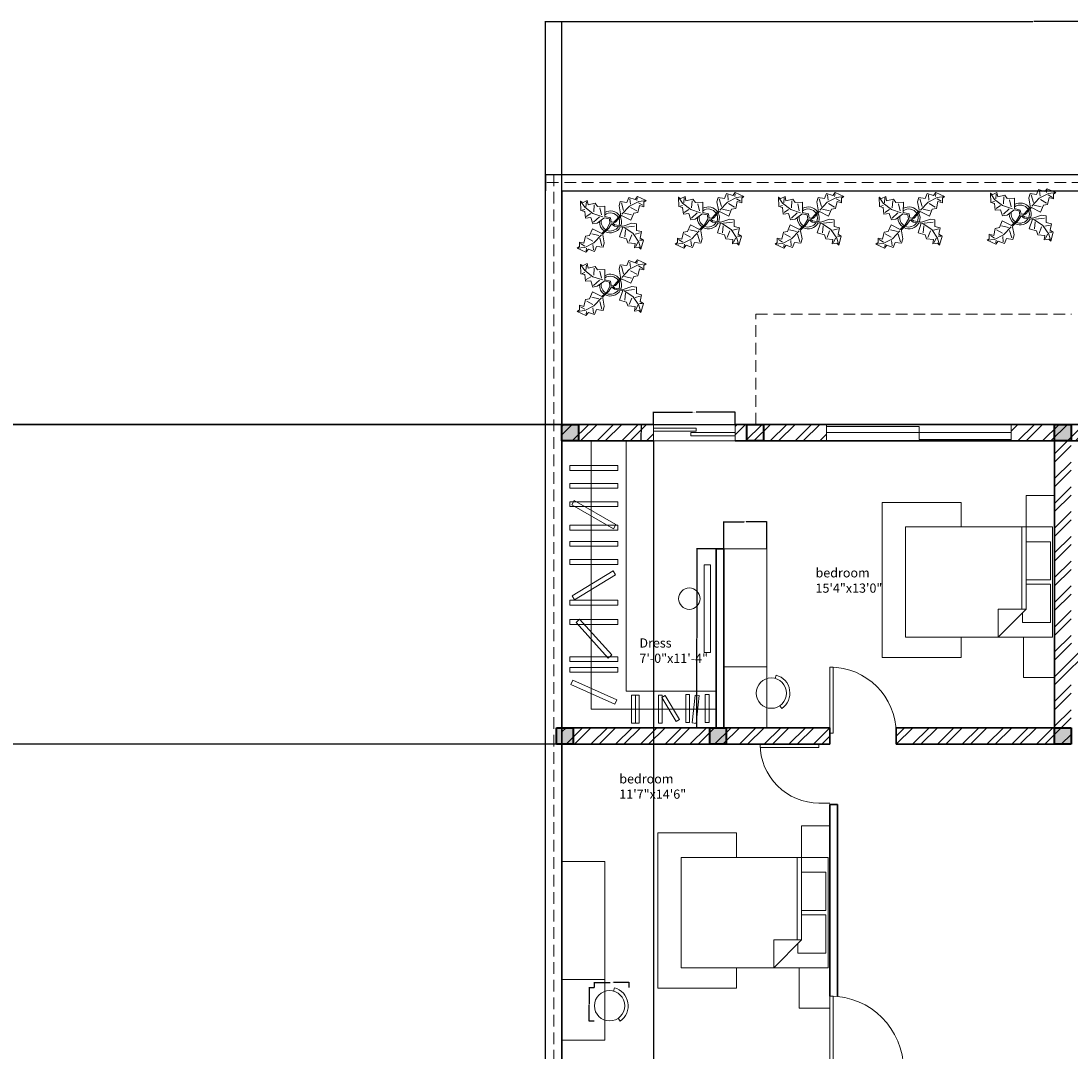
# Model space of a CAD drawing. Units: inches. Extents: x 19613 to 21413, y 12082 to 13202.
# Tile 8 of 9: x 20513 to 21084, y 12641 to 13202. Entities that reach past the tile are written whole.
import ezdxf

# ---------------------------------------------------------------- set-up
doc = ezdxf.new("R2010")
doc.units = ezdxf.units.IN
doc.linetypes.add('HIDDEN', pattern=[9.525, 6.35, -3.175])
for name, color, linetype, lineweight in [('A-ANNO-DIMS', 2, 'Continuous', 18), ('A-AREA-IDEN', 7, 'Continuous', 18), ('A-COLS', 7, 'Continuous', 40), ('A-COLS-PATT', 6, 'Continuous', 13), ('A-DOOR', 3, 'Continuous', 18), ('A-FLOR-CASE', 9, 'Continuous', 18), ('A-FLOR-HIDN', 8, 'HIDDEN', 13), ('A-FURN', 8, 'Continuous', 18), ('A-GLAZ', 4, 'Continuous', 18), ('A-WALL', 7, 'Continuous', 35), ('A-WALL-PATT', 252, 'Continuous', 13), ('C-PROP', 7, 'Continuous', 25), ('C-PROP-HIDN', 8, 'HIDDEN', 13), ('L-PLNT', 116, 'Continuous', 18)]:
    doc.layers.add(name, color=color, linetype=linetype, lineweight=lineweight)
doc.styles.get("Standard").update_dxf_attribs({"font": 'arial.ttf'})
doc.dimstyles.get("Standard").update_dxf_attribs({"dimtxt": 0.18, "dimasz": 0.18, "dimexe": 0.18, "dimexo": 0.0625, "dimgap": 0.09, "dimtad": 0, "dimtih": 1, "dimtoh": 1, "dimdec": 4, "dimzin": 0, "dimdsep": 46, "dimtxsty": 'Standard', "dimcen": 0.09, "dimadec": 0, "dimazin": 0, "dimtfac": 1, "dimtdec": 4, "dimtofl": 0, "dimtmove": 0, "dimatfit": 3, "dimfxl": 1, "dimtolj": 1, "dimtzin": 0, "dimarcsym": 0})

# ---------------------------------------------------------------- blocks, each defined once
blk = doc.blocks.new('*U4')
for p, q in [((0, 0), (0, -6)), ((36, 0), (36, -6))]:
    blk.add_line(p, q)
blk.add_lwpolyline([(0, 0), (0, 36), (1.75, 36), (1.75, 0)], close=True)
blk.add_arc((0, 0), 36, 0, 90)
blk = doc.blocks.new('Bed - Queen')
for p, q in [((0, -80.00003), (0, 0)), ((0, 0), (59.99999, 0)), ((59.99999, 0), (59.99999, -80.00003)), ((7.99999, -1.2), (28.79998, -1.2)), ((7.99999, -14.4), (7.99999, -1.2)), ((28.79998, -1.2), (28.79998, -14.4)), ((31.19999, -1.2), (51.99999, -1.2)), ((31.19999, -14.4), (31.19999, -1.2)), ((51.99999, -1.2), (51.99999, -16.4)), ((0, -14.4), (44.8, -14.4)), ((44.8, -16.8), (0, -16.8)), ((59.99999, -29.6), (44.8, -14.4)), ((44.8, -14.4), (44.8, -29.6)), ((51.99999, -16.4), (46.79936, -16.4)), ((44.8, -29.6), (59.99999, -29.6)), ((59.99999, -80.00003), (0, -80.00003))]:
    blk.add_line(p, q)
blk = doc.blocks.new('*U6')
for p, q in [((0, 0), (0, -6)), ((40, 0), (40, -6))]:
    blk.add_line(p, q)
blk.add_lwpolyline([(0, 0), (0, 40), (1.75, 40), (1.75, 0)], close=True)
blk.add_arc((0, 0), 40, 0, 90)
blk = doc.blocks.new('Plant - Rubber or Philodendron')
for p, q in [((-16.2005, 11.4774), (-13.9899, 8.1064)), ((-16.2005, 11.4774), (-14.8639, 10.7964)), ((-16.0159, 6.3329), (-16.2005, 11.4774)), ((-14.8639, 10.7964), (-12.6195, 11.8975)), ((-12.6195, 11.8975), (-12.1909, 9.4345)), ((8.8871, 10.7908), (9.9809, 13.4933)), ((9.9809, 13.4933), (13.3837, 12.301)), ((10.5828, 12.6946), (10.8893, 9.7953)), ((13.3837, 12.301), (14.68, 13.9039)), ((14.5816, 13.2037), (14.3848, 11.8033)), ((14.68, 13.9039), (19.3848, 11.8146)), ((19.3848, 11.8146), (15.3859, 11.3055)), ((19.3848, 11.8146), (18.1868, 10.9119)), ((-14.0069, 5.8704), (-16.0159, 6.3329)), ((-15.3434, 6.5514), (-13.9984, 6.9884)), ((-13.5868, 2.2894), (-14.0069, 5.8704)), ((-13.9899, 8.1064), (-9.5434, 4.7185)), ((-13.3174, 8.325), (-13.0735, 11.0065)), ((-12.1909, 9.4345), (-8.3829, 10.3)), ((-8.8369, 9.409), (-9.0894, 5.6095)), ((-8.3829, 10.3), (-7.0549, 8.501)), ((-7.0549, 8.501), (-3.0284, 8.6941)), ((-4.8529, 4.012), (-5.7184, 7.82)), ((-3.0284, 8.6941), (-3.0709, 3.1041)), ((4.6914, 8.8812), (5.3859, 11.2828)), ((4.6914, 8.8812), (5.5014, 4.4831)), ((5.3859, 11.2828), (8.8871, 10.7908)), ((5.9878, 10.4842), (7.1971, 6.3869)), ((10.3916, 8.7942), (6.2847, 4.4028)), ((15.3859, 11.3055), (10.3916, 8.7942)), ((14.2977, 6.1031), (10.9934, 7.9956)), ((15.7909, 9.1065), (14.8995, 5.3044)), ((15.2875, 10.6053), (17.5907, 9.2105)), ((18.1925, 8.4119), (15.7909, 9.1065)), ((18.1868, 10.9119), (18.1925, 8.4119)), ((-10.6784, 2.491), (-13.5868, 2.2894)), ((-13.1329, 3.1804), (-10.6614, 4.727)), ((-9.5858, -0.8715), (-10.6784, 2.491)), ((-9.5434, 4.7185), (-4.1917, 2.9888)), ((-9.1318, 0.0195), (-5.9793, 2.9025)), ((-7.1228, -0.443), (-3.5248, 2.2131)), ((-3.5248, 2.2131), (-3.3011, 2.4355)), ((-3.3011, 2.4355), (-0.5306, 1.7947)), ((-3.0709, 3.1041), (0.0797, 2.3163)), ((-0.5306, 1.7947), (-0.2255, -0.5527)), ((-0.5306, 1.7947), (-0.5306, 1.7947)), ((0.0797, 2.3163), (0.4866, -0.031)), ((0.4866, -0.031), (2.1141, 0.2298)), ((2.1141, 0.2298), (5.4346, 3.9146)), ((6.1032, 3.6844), (2.8262, -0.031)), ((5.4346, 3.9146), (5.5014, 4.4831)), ((11.1089, 1.1958), (6.1032, 3.6844)), ((7.7005, 4.8881), (11.5025, 3.9967)), ((12.7005, 4.8994), (11.1089, 1.1958)), ((14.8995, 5.3044), (12.7005, 4.8994)), ((-11.3237, -7.2629), (-9.7321, -3.5593)), ((-9.7321, -3.5593), (-4.7264, -6.0479)), ((-7.1228, -0.443), (-9.5858, -0.8715)), ((-2.019, -3.6148), (-4.7264, -6.0479)), ((-4.0579, -6.2781), (-0.9375, -3.1608)), ((-2.019, -3.6148), (-0.2255, -0.5527)), ((-0.9375, -3.1608), (0.5883, -0.8135)), ((0.5883, -0.8135), (2.2447, -2.0916)), ((2.8262, -0.031), (1.3003, -0.5527)), ((1.3003, -0.5527), (2.4193, -1.4655)), ((2.2447, -2.0916), (6.7108, -2.6626)), ((2.4193, -1.4655), (6.895, -2.1175)), ((4.943, -7.9659), (6.7108, -2.6626)), ((11.6605, -0.5413), (6.895, -2.1175)), ((12.3677, -6.1981), (7.219, -2.6772)), ((8.125, -4.0768), (7.7715, -7.9659)), ((8.3544, -2.7453), (13.1973, -2.1704)), ((11.6605, -0.5413), (14.1354, -0.8948)), ((14.1354, -0.8948), (14.1354, -4.4304)), ((14.1354, -4.4304), (16.9638, -5.1375)), ((16.9638, -5.1375), (16.2567, -8.673)), ((-16.8157, -10.7754), (-14.4141, -11.4699)), ((-16.8101, -13.2754), (-16.8157, -10.7754)), ((-14.4141, -11.4699), (-13.5228, -7.6679)), ((-14.0091, -13.669), (-9.0148, -11.1577)), ((-13.5228, -7.6679), (-11.3237, -7.2629)), ((-12.921, -8.4665), (-9.6166, -10.359)), ((-6.3237, -7.2516), (-10.1257, -6.3602)), ((-9.0148, -11.1577), (-4.9047, -6.8122)), ((-4.611, -12.8477), (-5.8203, -8.7504)), ((-4.1246, -6.8466), (-4.0579, -6.2781)), ((-3.3146, -11.2447), (-4.1246, -6.8466)), ((-3.3146, -11.2447), (-4.0092, -13.6463)), ((8.8321, -9.0266), (4.943, -7.9659)), ((9.5392, -11.1479), (8.8321, -9.0266)), ((13.4283, -11.5015), (9.5392, -11.1479)), ((10.2463, -10.4408), (11.6605, -6.9053)), ((15.5496, -10.7943), (12.3677, -6.1981)), ((16.2567, -5.8446), (13.4283, -6.5517)), ((14.8425, -10.7943), (13.7819, -13.2692)), ((16.6103, -14.6834), (15.5496, -10.7943)), ((17.3174, -9.7337), (15.9032, -9.7337)), ((16.2567, -8.673), (18.0245, -9.7337)), ((18.0245, -9.7337), (16.6103, -14.6834)), ((-18.008, -14.1781), (-16.8101, -13.2754)), ((-18.008, -14.1781), (-14.0091, -13.669)), ((-13.3032, -16.2674), (-18.008, -14.1781)), ((-13.9107, -12.9688), (-16.2139, -11.574)), ((-12.0069, -14.6645), (-13.3032, -16.2674)), ((-13.2048, -15.5672), (-13.008, -14.1668)), ((-8.6042, -15.8568), (-12.0069, -14.6645)), ((-9.206, -15.0581), (-9.5126, -12.1588)), ((-7.5103, -13.1543), (-8.6042, -15.8568)), ((-4.0092, -13.6463), (-7.5103, -13.1543)), ((13.0748, -13.9763), (13.4283, -11.5015)), ((15.5496, -13.6228), (13.0748, -13.9763)), ((16.6103, -14.6834), (15.5496, -13.6228))]:
    blk.add_line(p, q)
for centre, radius, start, end in [((0, 0), 6.1275, 34.37569, 120.1028), ((0.0308, 0.1664), 6, 178.6147, 235.1169), ((0.0308, 0.1664), 5, 168.1647, 238.6725), ((-0.0601, -0.2075), 5.2461, 33.82192, 124.9414), ((-0.2664, 0.1682), 5.2775, 338.4094, 20.03007), ((-0.098, 0.1364), 6.1288, 341.2017, 26.09184), ((-0.0234, 0.3825), 6.1492, 242.5812, 331.2714), ((-0.1102, 0.4886), 5.2883, 247.3711, 327.472)]:
    blk.add_arc(centre, radius, start, end)
blk = doc.blocks.new('*U16')
for p, q in [((0, 0), (0, 6)), ((32, 0), (32, 6))]:
    blk.add_line(p, q)
blk.add_lwpolyline([(0, 0), (0, -32), (1.75, -32), (1.75, 0)], close=True)
blk.add_arc((0, 0), 32, 270, 0)
blk = doc.blocks.new('COL-9x9')
for p, q in [((0, 9), (9, 9)), ((0, 0), (0, 9)), ((9, 9), (9, 0)), ((9, 0), (0, 0))]:
    blk.add_line(p, q)
blk = doc.blocks.new('CLOSET-L-RAIL')
for p, q in [((11.57, 153.64), (11.57, 7.7)), ((30.65, 153.64), (30.65, 17.54)), ((30.65, 17.54), (79.7, 17.54)), ((11.57, 7.7), (79.7, 7.7))]:
    blk.add_line(p, q)
for points in [[(0, 140.24), (26.12, 140.24), (26.12, 137.64), (0, 137.64)], [(0, 130.54), (26.12, 130.54), (26.12, 127.95), (0, 127.95)], [(0, 120.52), (26.12, 120.52), (26.12, 117.92), (0, 117.92)], [(2.39, 121.15), (25.03, 108.13), (23.74, 105.88), (1.09, 118.9)], [(0, 107.73), (26.12, 107.73), (26.12, 105.13), (0, 105.13)], [(0, 98.91), (26.12, 98.91), (26.12, 96.32), (0, 96.32)], [(0, 89.07), (26.12, 89.07), (26.12, 86.48), (0, 86.48)], [(1.22, 69.39), (23.56, 82.95), (24.9, 80.73), (2.57, 67.18)], [(0, 66.96), (26.12, 66.96), (26.12, 64.37), (0, 64.37)], [(0, 56.45), (26.12, 56.45), (26.12, 53.86), (0, 53.86)], [(5.27, 56.6), (22.78, 37.21), (20.85, 35.47), (3.35, 54.86)], [(0, 36.27), (26.12, 36.27), (26.12, 33.68), (0, 33.68)], [(0, 30.47), (26.12, 30.47), (26.12, 27.88), (0, 27.88)], [(1.67, 23.53), (25.51, 12.85), (24.45, 10.49), (0.61, 21.17)], [(35.67, 0.07), (33.61, 0.07), (33.61, 15.33), (35.67, 15.33)], [(37.73, 0.07), (35.67, 0.07), (35.67, 15.33), (37.73, 15.33)], [(50.3, 0.07), (48.24, 0.07), (48.24, 15.33), (50.3, 15.33)], [(59.69, 2.02), (57.92, 0.97), (50.13, 14.1), (51.9, 15.15)], [(65.15, 0.43), (63.09, 0.43), (63.09, 15.69), (65.15, 15.69)], [(68.26, 15.4), (70.31, 15.18), (68.65, 0), (66.6, 0.22)], [(75.77, 0.43), (73.71, 0.43), (73.71, 15.69), (75.77, 15.69)]]:
    blk.add_lwpolyline(points, close=True)
blk = doc.blocks.new('WINDOW-BEDROOM-SLIDER')
for p, q in [((0, 9), (0, 0)), ((0, 9), (100.32, 9)), ((0, 0), (0, 9)), ((50.28, 7.85), (0, 7.85)), ((50.28, 4.5), (50.28, 7.85)), ((50.28, 7.85), (50.28, 4.5)), ((100.32, 9), (100.32, 0)), ((100.32, 9), (100.32, 0.84)), ((0, 4.5), (50.28, 4.5)), ((50.28, 4.5), (100.32, 4.5)), ((100.32, 4.5), (50.28, 4.5)), ((50.28, 4.5), (50.28, 0.84)), ((50.28, 0.84), (100.32, 0.84)), ((100.32, 0.84), (100.32, 0)), ((100.32, 0), (0, 0))]:
    blk.add_line(p, q)
blk = doc.blocks.new('WINDOW-DRESS-SLIDER')
for p, q in [((0, 9), (0, 0)), ((0, 9), (44.45, 9)), ((44.45, 9), (44.45, 0)), ((0, 0), (44.45, 0))]:
    blk.add_line(p, q)
for points in [[(0, 6.95), (23.27, 6.95), (23.27, 5.37), (0, 5.37)], [(44.45, 4.5), (20.22, 4.5), (20.22, 2.83), (44.45, 2.83)]]:
    blk.add_lwpolyline(points, close=True)
blk = doc.blocks.new('DESK-CHAIR-ROUND')
for p, q in [((10.85, 18.16), (10.37, 16.34)), ((13.96, 0), (12.89, 1.56))]:
    blk.add_line(p, q)
blk.add_circle((8.25, 8.37), 8.25)
blk.add_arc((8.25, 8.37), 10.13, 304.3105, 75.0908)
blk = doc.blocks.new('BEDROOM-DESK-SLIM')
for p, q in [((0, 97.32), (23.4, 97.32)), ((23.4, 97.32), (23.4, 0)), ((0, 33.03), (23.4, 33.03))]:
    blk.add_line(p, q)
blk = doc.blocks.new('BEDROOM-AREA-RUG')
for p, q in [((42.96, 84.39), (0, 84.39)), ((0, 84.39), (0, 0)), ((42.96, 71.03), (42.96, 84.39)), ((12.72, 71.03), (42.96, 71.03)), ((42.96, 0), (42.96, 11.03)), ((0, 0), (42.96, 0))]:
    blk.add_line(p, q)
blk = doc.blocks.new('*D45')
at = {"layer": 'A-ANNO-DIMS', "color": 0, "lineweight": -2, "transparency": 16777216}
for p, q in [((20825.11, 12675.88), (20825.11, 12678.83)), ((20844.01, 12675.88), (20844.01, 12678.83)), ((20825.29, 12678.65), (20833.6, 12678.65)), ((20843.83, 12678.65), (20835.51, 12678.65))]:
    blk.add_line(p, q, dxfattribs=at)
at = {"layer": 'A-ANNO-DIMS', "color": 0, "transparency": 16777216}
for points in [[(20825.29, 12678.68), (20825.29, 12678.62), (20825.11, 12678.65)], [(20843.83, 12678.68), (20843.83, 12678.62), (20844.01, 12678.65)]]:
    blk.add_solid(points, dxfattribs=at)
at = {"layer": 'Defpoints', "color": 0, "transparency": 16777216}
for p in [(20825.11, 12675.81), (20844.01, 12678.65), (20844.01, 12675.81)]:
    blk.add_point(p, dxfattribs=at)
at = {"layer": 'A-ANNO-DIMS', "color": 0, "transparency": 16777216, "insert": (20834.56, 12678.65), "char_height": 0.18, "attachment_point": 5}
blk.add_mtext('\\A1;CHAIR 19 TYP.', dxfattribs=at)
blk = doc.blocks.new('*D46')
at = {"layer": 'A-ANNO-DIMS', "color": 0, "lineweight": -2, "transparency": 16777216}
for p, q in [((20825.04, 12675.81), (20822.09, 12675.81)), ((20822.27, 12675.63), (20822.27, 12666.92)), ((20822.27, 12657.83), (20822.27, 12666.55)), ((20825.04, 12657.65), (20822.09, 12657.65))]:
    blk.add_line(p, q, dxfattribs=at)
at = {"layer": 'A-ANNO-DIMS', "color": 0, "transparency": 16777216}
for points in [[(20822.24, 12675.63), (20822.3, 12675.63), (20822.27, 12675.81)], [(20822.24, 12657.83), (20822.3, 12657.83), (20822.27, 12657.65)]]:
    blk.add_solid(points, dxfattribs=at)
at = {"layer": 'Defpoints', "color": 0, "transparency": 16777216}
for p in [(20822.27, 12675.81), (20825.11, 12675.81), (20825.11, 12657.65)]:
    blk.add_point(p, dxfattribs=at)
at = {"layer": 'A-ANNO-DIMS', "color": 0, "transparency": 16777216, "insert": (20822.27, 12666.73), "char_height": 0.18, "attachment_point": 5}
blk.add_mtext('\\A1;18 TYP.', dxfattribs=at)
blk = doc.blocks.new('*D47')
at = {"layer": 'A-ANNO-DIMS', "color": 0, "lineweight": -2, "transparency": 16777216}
for p, q in [((20895.37, 12914.6), (20880.66, 12914.6)), ((20880.84, 12914.42), (20880.84, 12866.12)), ((20880.84, 12817.46), (20880.84, 12865.75)), ((20895.37, 12817.28), (20880.66, 12817.28))]:
    blk.add_line(p, q, dxfattribs=at)
at = {"layer": 'A-ANNO-DIMS', "color": 0, "transparency": 16777216}
for points in [[(20880.81, 12914.42), (20880.87, 12914.42), (20880.84, 12914.6)], [(20880.81, 12817.46), (20880.87, 12817.46), (20880.84, 12817.28)]]:
    blk.add_solid(points, dxfattribs=at)
at = {"layer": 'Defpoints', "color": 0, "transparency": 16777216}
for p in [(20880.84, 12914.6), (20895.43, 12914.6), (20895.43, 12817.28)]:
    blk.add_point(p, dxfattribs=at)
at = {"layer": 'A-ANNO-DIMS', "color": 0, "transparency": 16777216, "insert": (20880.84, 12865.94), "char_height": 0.18, "attachment_point": 5}
blk.add_mtext('\\A1;DESK 97 TYP.', dxfattribs=at)
blk = doc.blocks.new('*D48')
at = {"layer": 'A-ANNO-DIMS', "color": 0, "lineweight": -2, "transparency": 16777216}
for p, q in [((20895.43, 12914.66), (20895.43, 12929.37)), ((20895.61, 12929.19), (20906.6, 12929.19)), ((20918.65, 12929.19), (20907.66, 12929.19)), ((20918.83, 12914.66), (20918.83, 12929.37))]:
    blk.add_line(p, q, dxfattribs=at)
at = {"layer": 'A-ANNO-DIMS', "color": 0, "transparency": 16777216}
for points in [[(20895.61, 12929.22), (20895.61, 12929.16), (20895.43, 12929.19)], [(20918.65, 12929.22), (20918.65, 12929.16), (20918.83, 12929.19)]]:
    blk.add_solid(points, dxfattribs=at)
at = {"layer": 'Defpoints', "color": 0, "transparency": 16777216}
for p in [(20918.83, 12929.19), (20895.43, 12914.6), (20918.83, 12914.6)]:
    blk.add_point(p, dxfattribs=at)
at = {"layer": 'A-ANNO-DIMS', "color": 0, "transparency": 16777216, "insert": (20907.13, 12929.19), "char_height": 0.18, "attachment_point": 5}
blk.add_mtext('\\A1;23 TYP.', dxfattribs=at)
blk = doc.blocks.new('*D63')
at = {"layer": 'A-ANNO-DIMS', "color": 0, "lineweight": -2, "transparency": 16777216}
for p, q in [((20857.28, 12982.34), (20857.28, 12989.13)), ((20857.46, 12988.95), (20878.49, 12988.95)), ((20901.55, 12988.95), (20880.52, 12988.95)), ((20901.73, 12982.34), (20901.73, 12989.13))]:
    blk.add_line(p, q, dxfattribs=at)
at = {"layer": 'A-ANNO-DIMS', "color": 0, "transparency": 16777216}
for points in [[(20857.46, 12988.98), (20857.46, 12988.92), (20857.28, 12988.95)], [(20901.55, 12988.98), (20901.55, 12988.92), (20901.73, 12988.95)]]:
    blk.add_solid(points, dxfattribs=at)
at = {"layer": 'Defpoints', "color": 0, "transparency": 16777216}
for p in [(20901.73, 12988.95), (20857.28, 12982.28), (20901.73, 12982.28)]:
    blk.add_point(p, dxfattribs=at)
at = {"layer": 'A-ANNO-DIMS', "color": 0, "transparency": 16777216, "insert": (20879.5, 12988.95), "char_height": 0.18, "attachment_point": 5}
blk.add_mtext('\\A1;SLIDER 44 TYP.', dxfattribs=at)
blk = doc.blocks.new('*D64')
at = {"layer": 'A-ANNO-DIMS', "color": 0, "lineweight": -2, "transparency": 16777216}
for p, q in [((20857.22, 12982.28), (20850.43, 12982.28)), ((20850.61, 12982.1), (20850.61, 12977.96)), ((20850.61, 12973.46), (20850.61, 12977.6)), ((20857.22, 12973.28), (20850.43, 12973.28))]:
    blk.add_line(p, q, dxfattribs=at)
at = {"layer": 'A-ANNO-DIMS', "color": 0, "transparency": 16777216}
for points in [[(20850.58, 12982.1), (20850.64, 12982.1), (20850.61, 12982.28)], [(20850.58, 12973.46), (20850.64, 12973.46), (20850.61, 12973.28)]]:
    blk.add_solid(points, dxfattribs=at)
at = {"layer": 'Defpoints', "color": 0, "transparency": 16777216}
for p in [(20850.61, 12982.28), (20857.28, 12982.28), (20857.28, 12973.28)]:
    blk.add_point(p, dxfattribs=at)
at = {"layer": 'A-ANNO-DIMS', "color": 0, "transparency": 16777216, "insert": (20850.61, 12977.78), "char_height": 0.18, "attachment_point": 5}
blk.add_mtext('\\A1;9 TYP.', dxfattribs=at)
blk = doc.blocks.new('*D85')
at = {"layer": 'A-ANNO-DIMS', "color": 0, "lineweight": -2, "transparency": 16777216}
for p, q in [((20798.43, 13118.34), (20798.43, 13201.71)), ((20798.61, 13201.53), (21063.66, 13201.53)), ((21329.25, 13201.53), (21064.21, 13201.53)), ((21329.43, 13118.34), (21329.43, 13201.71))]:
    blk.add_line(p, q, dxfattribs=at)
at = {"layer": 'A-ANNO-DIMS', "color": 0, "transparency": 16777216}
for points in [[(20798.61, 13201.56), (20798.61, 13201.5), (20798.43, 13201.53)], [(21329.25, 13201.56), (21329.25, 13201.5), (21329.43, 13201.53)]]:
    blk.add_solid(points, dxfattribs=at)
at = {"layer": 'Defpoints', "color": 0, "transparency": 16777216}
for p in [(21329.43, 13201.53), (20798.43, 13118.28), (21329.43, 13118.28)]:
    blk.add_point(p, dxfattribs=at)
at = {"layer": 'A-ANNO-DIMS', "color": 0, "transparency": 16777216, "insert": (21063.93, 13201.53), "char_height": 0.18, "attachment_point": 5}
blk.add_mtext('\\A1;531', dxfattribs=at)
blk = doc.blocks.new('*D87')
at = {"layer": 'A-ANNO-DIMS', "color": 0, "lineweight": -2, "transparency": 16777216}
for p, q in [((20218.76, 12982.28), (21412.86, 12982.28)), ((21412.68, 12982.1), (21412.68, 12697.46)), ((21412.68, 12412.46), (21412.68, 12697.1)), ((20218.76, 12412.28), (21412.86, 12412.28))]:
    blk.add_line(p, q, dxfattribs=at)
at = {"layer": 'A-ANNO-DIMS', "color": 0, "transparency": 16777216}
for points in [[(21412.65, 12982.1), (21412.71, 12982.1), (21412.68, 12982.28)], [(21412.65, 12412.46), (21412.71, 12412.46), (21412.68, 12412.28)]]:
    blk.add_solid(points, dxfattribs=at)
at = {"layer": 'Defpoints', "color": 0, "transparency": 16777216}
for p in [(20218.69, 12982.28), (21412.68, 12982.28), (20218.69, 12412.28)]:
    blk.add_point(p, dxfattribs=at)
at = {"layer": 'A-ANNO-DIMS', "color": 0, "transparency": 16777216, "insert": (21412.68, 12697.28), "char_height": 0.18, "attachment_point": 5}
blk.add_mtext('\\A1;570', dxfattribs=at)
blk = doc.blocks.new('*D89')
at = {"layer": 'A-ANNO-DIMS', "color": 0, "lineweight": -2, "transparency": 16777216}
for p, q in [((20807.37, 12808.28), (19613.26, 12808.28)), ((19613.44, 12808.1), (19613.44, 12721.46)), ((19613.44, 12634.46), (19613.44, 12721.1)), ((20807.37, 12634.28), (19613.26, 12634.28))]:
    blk.add_line(p, q, dxfattribs=at)
at = {"layer": 'A-ANNO-DIMS', "color": 0, "transparency": 16777216}
for points in [[(19613.41, 12808.1), (19613.47, 12808.1), (19613.44, 12808.28)], [(19613.41, 12634.46), (19613.47, 12634.46), (19613.44, 12634.28)]]:
    blk.add_solid(points, dxfattribs=at)
at = {"layer": 'Defpoints', "color": 0, "transparency": 16777216}
for p in [(19613.44, 12808.28), (20807.43, 12808.28), (20807.43, 12634.28)]:
    blk.add_point(p, dxfattribs=at)
at = {"layer": 'A-ANNO-DIMS', "color": 0, "transparency": 16777216, "insert": (19613.44, 12721.28), "char_height": 0.18, "attachment_point": 5}
blk.add_mtext('\\A1;174', dxfattribs=at)
blk = doc.blocks.new('*D90')
at = {"layer": 'A-ANNO-DIMS', "color": 0, "lineweight": -2, "transparency": 16777216}
for p, q in [((20807.37, 12982.28), (19613.26, 12982.28)), ((19613.44, 12982.1), (19613.44, 12895.46)), ((19613.44, 12808.46), (19613.44, 12895.1)), ((20807.37, 12808.28), (19613.26, 12808.28))]:
    blk.add_line(p, q, dxfattribs=at)
at = {"layer": 'A-ANNO-DIMS', "color": 0, "transparency": 16777216}
for points in [[(19613.41, 12982.1), (19613.47, 12982.1), (19613.44, 12982.28)], [(19613.41, 12808.46), (19613.47, 12808.46), (19613.44, 12808.28)]]:
    blk.add_solid(points, dxfattribs=at)
at = {"layer": 'Defpoints', "color": 0, "transparency": 16777216}
for p in [(19613.44, 12982.28), (20807.43, 12982.28), (20807.43, 12808.28)]:
    blk.add_point(p, dxfattribs=at)
at = {"layer": 'A-ANNO-DIMS', "color": 0, "transparency": 16777216, "insert": (19613.44, 12895.28), "char_height": 0.18, "attachment_point": 5}
blk.add_mtext('\\A1;174', dxfattribs=at)
blk = doc.blocks.new('*D98')
at = {"layer": 'A-ANNO-DIMS', "color": 0, "lineweight": -2, "transparency": 16777216}
for p, q in [((20807.43, 12982.34), (20807.43, 13201.71)), ((20807.61, 13201.53), (21063.64, 13201.53)), ((21320.25, 13201.53), (21064.22, 13201.53)), ((21320.43, 12982.34), (21320.43, 13201.71))]:
    blk.add_line(p, q, dxfattribs=at)
at = {"layer": 'A-ANNO-DIMS', "color": 0, "transparency": 16777216}
for points in [[(20807.61, 13201.56), (20807.61, 13201.5), (20807.43, 13201.53)], [(21320.25, 13201.56), (21320.25, 13201.5), (21320.43, 13201.53)]]:
    blk.add_solid(points, dxfattribs=at)
at = {"layer": 'Defpoints', "color": 0, "transparency": 16777216}
for p in [(21320.43, 13201.53), (20807.43, 12982.28), (21320.43, 12982.28)]:
    blk.add_point(p, dxfattribs=at)
at = {"layer": 'A-ANNO-DIMS', "color": 0, "transparency": 16777216, "insert": (21063.93, 13201.53), "char_height": 0.18, "attachment_point": 5}
blk.add_mtext('\\A1;513', dxfattribs=at)
blk = doc.blocks.new('*D100')
at = {"layer": 'A-ANNO-DIMS', "color": 0, "lineweight": -2, "transparency": 16777216}
for p, q in [((20807.43, 12973.22), (20807.43, 12091.85)), ((20857.28, 12973.22), (20857.28, 12091.85)), ((20807.61, 12092.03), (20831.96, 12092.03)), ((20857.1, 12092.03), (20832.75, 12092.03))]:
    blk.add_line(p, q, dxfattribs=at)
at = {"layer": 'A-ANNO-DIMS', "color": 0, "transparency": 16777216}
for points in [[(20807.61, 12092.06), (20807.61, 12092), (20807.43, 12092.03)], [(20857.1, 12092.06), (20857.1, 12092), (20857.28, 12092.03)]]:
    blk.add_solid(points, dxfattribs=at)
at = {"layer": 'Defpoints', "color": 0, "transparency": 16777216}
for p in [(20807.43, 12973.28), (20857.28, 12973.28), (20857.28, 12092.03)]:
    blk.add_point(p, dxfattribs=at)
at = {"layer": 'A-ANNO-DIMS', "color": 0, "transparency": 16777216, "insert": (20832.36, 12092.03), "char_height": 0.18, "attachment_point": 5}
blk.add_mtext('\\A1;49.85', dxfattribs=at)

msp = doc.modelspace()

# ---------------------------------------------------------------- hatches: boundary and pattern name
at = {"layer": 'A-COLS-PATT'}
h = msp.add_hatch(color=256, dxfattribs=at)
h.dxf.hatch_style = 1
h.paths.add_polyline_path([(20816.4328, 12982.279), (20807.4339, 12982.279), (20807.4339, 12973.279), (20816.4328, 12973.279)])
h.paths.add_polyline_path([(21084.4339, 12982.279), (21075.4339, 12982.279), (21075.4339, 12973.279), (21084.4339, 12973.279)])
h.paths.add_polyline_path([(21320.4339, 12982.279), (21311.4729, 12982.279), (21311.4729, 12973.279), (21320.4339, 12973.279)])
h.paths.add_polyline_path([(21320.3201, 12808.279), (21311.3201, 12808.279), (21311.3201, 12803.279), (21320.3201, 12803.279)])
h.paths.add_polyline_path([(21320.3201, 12812.279), (21311.3201, 12812.279), (21311.3201, 12808.279), (21320.3201, 12808.279)])
h.paths.add_polyline_path([(21320.3574, 12634.279), (21311.3574, 12634.279), (21311.3574, 12625.279), (21320.3574, 12625.279)])
h.paths.add_polyline_path([(21319.9035, 12421.1076), (21310.9035, 12421.1076), (21310.9035, 12412.279), (21319.9035, 12412.279)])
h.paths.add_polyline_path([(21086.1238, 12454.2407), (21077.1238, 12454.2407), (21077.1238, 12445.279), (21077.4339, 12445.279), (21086.1238, 12445.279)])
h.paths.add_polyline_path([(21014.4339, 12454.2407), (21005.4339, 12454.2407), (21005.4339, 12445.279), (21014.4339, 12445.279)])
h.paths.add_polyline_path([(21014.3637, 12634.279), (21005.3637, 12634.279), (21005.3637, 12625.5213), (21014.3637, 12625.5213)])
h.paths.add_polyline_path([(21086.4339, 12634.279), (21077.4339, 12634.279), (21077.4339, 12625.5213), (21086.4339, 12625.5213)])
h.paths.add_polyline_path([(20814.1423, 12634.279), (20807.4339, 12634.279), (20807.4339, 12625.4792), (20814.1423, 12625.4792)])
h.paths.add_polyline_path([(20807.4339, 12634.279), (20807.4339, 12634.4792), (20805.1423, 12634.4792), (20805.1423, 12625.4792), (20807.4339, 12625.4792)])
h.paths.add_polyline_path([(20807.4339, 12439.1296), (20802.9339, 12439.1296), (20802.9339, 12430.1296), (20807.4339, 12430.1296)])
h.paths.add_polyline_path([(20802.9339, 12439.1296), (20798.4339, 12439.1296), (20798.4339, 12430.1296), (20802.9339, 12430.1296)])
h.paths.add_polyline_path([(20813.4646, 12817.279), (20807.4339, 12817.279), (20807.4339, 12808.279), (20813.4646, 12808.279)])
h.paths.add_polyline_path([(20807.4339, 12817.279), (20804.4646, 12817.279), (20804.4646, 12808.279), (20807.4339, 12808.279)])
h.paths.add_polyline_path([(20896.8418, 12817.279), (20887.8418, 12817.279), (20887.8418, 12808.279), (20896.8418, 12808.279)])
h.paths.add_polyline_path([(21084.4339, 12817.279), (21075.4339, 12817.279), (21075.4339, 12808.279), (21084.4339, 12808.279)])
h.paths.add_polyline_path([(21201.8616, 12982.279), (21182.5788, 12982.279), (21182.5788, 12973.279), (21193.4339, 12973.279), (21201.8616, 12973.279), (21201.8616, 12976.279)])
at = {"layer": 'A-WALL-PATT'}
h = msp.add_hatch(dxfattribs=at)
h.set_pattern_fill('ANSI32', color=256)
h.paths.add_polyline_path([(20223.1937, 13118.279), (20218.6937, 13118.279), (19701.1937, 13118.279), (19701.1937, 13113.779), (20223.1937, 13113.779)])
h.paths.add_polyline_path([(19849.7315, 12982.279), (19799.9854, 12982.279), (19799.9854, 12973.279), (19849.7315, 12973.279)])
h.paths.add_polyline_path([(19755.5378, 12982.279), (19705.6937, 12982.279), (19705.6937, 12973.279), (19755.5378, 12973.279)])
h.paths.add_polyline_path([(20000.1054, 12982.279), (19950.0534, 12982.279), (19950.0534, 12974.1171), (19950.0534, 12973.279), (20000.1054, 12973.279)])
h.paths.add_polyline_path([(20049.4797, 12982.279), (20030.7476, 12982.279), (20030.7476, 12973.279), (20049.4797, 12973.279)])
h.paths.add_polyline_path([(20100.1214, 12982.279), (20080.8386, 12982.279), (20080.8386, 12973.279), (20100.1214, 12973.279), (20100.1214, 12976.279)])
h.paths.add_polyline_path([(20218.6937, 12982.279), (20167.6937, 12982.279), (20140.1214, 12982.279), (20140.1214, 12976.279, -0.01769781), (20140.0212, 12973.45), (20167.6937, 12973.279), (20176.6937, 12973.279), (20218.6937, 12973.279)])
h.paths.add_polyline_path([(19851.5503, 12814.279), (19851.5503, 12817.279), (19793.6937, 12817.279), (19789.6937, 12817.279), (19705.6937, 12817.279), (19705.6937, 12808.279), (19851.5503, 12808.279)])
h.paths.add_polyline_path([(19982.6937, 12973.279), (19973.6937, 12973.279), (19973.6937, 12817.279), (19887.5503, 12817.279), (19887.5503, 12808.279), (19973.6937, 12808.279), (19982.6937, 12808.279)])
h.paths.add_polyline_path([(20058.6937, 12850.5529), (19982.6937, 12850.5529), (19982.6937, 12846.5529), (20058.6937, 12846.5529)])
h.paths.add_polyline_path([(20095.6937, 12973.279), (20091.6937, 12973.279), (20091.6937, 12850.5529), (20087.6937, 12850.5529), (20087.6937, 12846.5529), (20095.6937, 12846.5529)])
h.paths.add_polyline_path([(20218.6937, 12808.279), (20140.8605, 12808.279), (20126.9413, 12808.279), (20126.9413, 12803.279), (20140.8605, 12803.279), (20218.6937, 12803.279)])
h.paths.add_polyline_path([(19738.3931, 12634.279), (19705.6937, 12634.279), (19705.6937, 12625.279), (19738.3931, 12625.279)])
h.paths.add_polyline_path([(19912.6937, 12634.279), (19903.6937, 12634.279), (19891.5503, 12634.279), (19891.5503, 12625.279), (19903.6937, 12625.279), (19903.6937, 12445.279), (19975.6937, 12445.279), (20128.6937, 12445.279), (20128.6937, 12412.279), (20149.8479, 12412.279), (20149.8479, 12421.279), (20137.6937, 12421.279), (20137.6937, 12454.279), (20137.6937, 12580.2801), (20133.6937, 12580.2801), (20133.6937, 12454.279), (19984.6937, 12454.279), (19984.6937, 12625.279), (19993.6937, 12625.279), (19993.6937, 12634.279), (19984.6937, 12634.279), (19975.6937, 12634.279), (19975.6937, 12454.279), (19912.6937, 12454.279)])
h.paths.add_polyline_path([(20218.6937, 12634.279), (20137.6937, 12634.279), (20029.6937, 12634.279), (20029.6937, 12625.279), (20137.6937, 12625.279), (20218.6937, 12625.279)])
h.paths.add_polyline_path([(21014.4339, 12634.279), (21005.4339, 12634.279), (20993.2905, 12634.279), (20993.2905, 12625.279), (21005.4339, 12625.279), (21005.4339, 12445.279), (21077.4339, 12445.279), (21230.4339, 12445.279), (21230.4339, 12412.279), (21251.5881, 12412.279), (21251.5881, 12421.279), (21239.4339, 12421.279), (21239.4339, 12454.279), (21239.4339, 12580.2801), (21235.4339, 12580.2801), (21235.4339, 12454.279), (21086.4339, 12454.279), (21086.4339, 12625.279), (21095.4339, 12625.279), (21095.4339, 12634.279), (21086.4339, 12634.279), (21077.4339, 12634.279), (21077.4339, 12454.279), (21014.4339, 12454.279)])
h.paths.add_polyline_path([(20840.1333, 12634.279), (20807.4339, 12634.279), (20807.4339, 12625.279), (20840.1333, 12625.279)])
h.paths.add_polyline_path([(20953.2905, 12631.279), (20953.2905, 12634.279), (20930.6216, 12634.279), (20930.6216, 12625.279), (20953.2905, 12625.279)])
h.paths.add_polyline_path([(21320.4339, 12634.279), (21239.4339, 12634.279), (21131.4339, 12634.279), (21131.4339, 12625.279), (21239.4339, 12625.279), (21320.4339, 12625.279)])
h.paths.add_polyline_path([(21084.4339, 12973.279), (21075.4339, 12973.279), (21075.4339, 12817.279), (20989.2905, 12817.279), (20989.2905, 12808.279), (21075.4339, 12808.279), (21084.4339, 12808.279)])
h.paths.add_polyline_path([(21142.1261, 12863.2893), (21084.4339, 12863.2893), (21084.4339, 12846.5529), (21142.1261, 12846.5529)])
h.paths.add_polyline_path([(21320.4339, 12808.279), (21242.6007, 12808.279), (21228.6815, 12808.279), (21228.6815, 12803.279), (21242.6007, 12803.279), (21320.4339, 12803.279)])
h.paths.add_polyline_path([(20857.278, 12982.279), (20807.4339, 12982.279), (20807.4339, 12973.279), (20857.278, 12973.279)])
h.paths.add_polyline_path([(20951.4717, 12982.279), (20901.7255, 12982.279), (20901.7255, 12973.279), (20951.4717, 12973.279)])
h.paths.add_polyline_path([(21101.8455, 12982.279), (21051.7936, 12982.279), (21051.7936, 12974.1171), (21051.7936, 12973.279), (21101.8455, 12973.279)])
h.paths.add_polyline_path([(21151.2199, 12982.279), (21132.4878, 12982.279), (21132.4878, 12973.279), (21151.2199, 12973.279)])
h.paths.add_polyline_path([(21201.8616, 12982.279), (21182.5788, 12982.279), (21182.5788, 12973.279), (21193.4339, 12973.279), (21201.8616, 12973.279), (21201.8616, 12976.279)])
h.paths.add_polyline_path([(21320.4339, 12982.279), (21269.4339, 12982.279), (21241.8616, 12982.279), (21241.8616, 12976.279, -0.01769781), (21241.7614, 12973.45), (21269.4339, 12973.279), (21278.4339, 12973.279), (21320.4339, 12973.279)])
h.paths.add_polyline_path([(20953.2905, 12817.279), (20895.4339, 12817.279), (20891.4339, 12817.279), (20807.4339, 12817.279), (20807.4339, 12808.279), (20953.2905, 12808.279)])
h.paths.add_polyline_path([(21197.4339, 12973.279), (21193.4339, 12973.279), (21193.4339, 12850.5529), (21197.4339, 12850.5529)])
h.paths.add_polyline_path([(21320.4339, 12550.279), (21272.5278, 12550.279), (21272.5278, 12546.279), (21320.4339, 12546.279)])
h.paths.add_polyline_path([(21320.4339, 12421.279), (21283.2222, 12421.279), (21283.2222, 12412.279), (21320.4339, 12412.279)])

# ---------------------------------------------------------------- linework, layer by layer
at = {"layer": 'A-FLOR-CASE'}
msp.add_lwpolyline([(20884.8298, 12905.912), (20888.2736, 12905.912), (20888.2736, 12858.2511), (20884.8298, 12858.2511)], close=True, dxfattribs=at)
msp.add_circle((20876.7223, 12887.4743), 5.828, dxfattribs=at)
at = {"layer": 'A-FLOR-HIDN'}
for p, q in [((20912.9732, 12982.279), (20912.9732, 13042.279)), ((20912.9732, 13042.279), (21084.6981, 13042.279))]:
    msp.add_line(p, q, dxfattribs=at)
at = {"layer": 'A-FURN'}
for p, q in [((21059.9903, 12926.479), (21059.9903, 12943.6155)), ((21059.9903, 12943.6155), (21075.4339, 12943.6155)), ((21058.6063, 12866.479), (21058.6063, 12844.5201)), ((21058.6063, 12844.5201), (21075.4339, 12844.5201)), ((20902.4847, 12760.0401), (20859.5277, 12760.0401)), ((20859.5277, 12760.0401), (20859.5277, 12675.6469)), ((20902.4847, 12746.6767), (20902.4847, 12760.0401)), ((20937.8469, 12746.6767), (20937.8469, 12763.8132)), ((20937.8469, 12763.8132), (20953.2905, 12763.8132)), ((20902.4847, 12675.6469), (20902.4847, 12686.6768)), ((20936.463, 12686.6768), (20936.463, 12664.7179)), ((20859.5277, 12675.6469), (20902.4847, 12675.6469)), ((20936.463, 12664.7179), (20953.2905, 12664.7179)), ((20830.8332, 12647.2306), (20807.4339, 12647.2306))]:
    msp.add_line(p, q, dxfattribs=at)
at = {"layer": 'A-WALL'}
for p, q in [((20857.278, 12982.279), (20807.4339, 12982.279)), ((21201.8616, 12982.279), (20901.7255, 12982.279)), ((20951.4717, 12982.279), (20987.6786, 12982.279)), ((20857.278, 12973.279), (20807.4339, 12973.279)), ((20807.4339, 12973.279), (20857.278, 12973.279)), ((21201.8616, 12973.279), (20901.7255, 12973.279)), ((20901.7255, 12973.279), (20951.4717, 12973.279)), ((21075.4339, 12973.279), (21084.4339, 12973.279)), ((20895.4339, 12914.5966), (20891.4339, 12914.5966)), ((20895.4339, 12817.279), (20895.4339, 12914.5966)), ((20807.4339, 12817.279), (20807.4339, 12808.279)), ((20891.4339, 12817.279), (20895.4339, 12817.279)), ((20895.4339, 12817.279), (20904.4339, 12817.279)), ((20895.4339, 12817.279), (20953.2905, 12817.279)), ((20953.2905, 12817.279), (20953.2905, 12808.279)), ((20989.2905, 12817.279), (20989.2905, 12808.279)), ((20807.4339, 12808.279), (20953.2905, 12808.279)), ((20807.4339, 12808.279), (20807.4339, 12634.279)), ((20989.2905, 12808.279), (21075.4339, 12808.279)), ((21084.4339, 12808.279), (21075.4339, 12808.279)), ((20953.2905, 12671.279), (20953.2905, 12775.4728)), ((20953.2905, 12775.4728), (20957.2905, 12775.4728)), ((20957.2905, 12671.279), (20957.2905, 12775.4728))]:
    msp.add_line(p, q, dxfattribs=at)
for points in [[(20891.4339, 12914.5966), (20891.4339, 12817.279), (20807.4339, 12817.279), (20807.4339, 12973.279), (20857.278, 12973.279)], [(20989.2905, 12817.279), (21075.4339, 12817.279), (21075.4339, 12973.279), (20901.7255, 12973.279)], [(20891.4339, 12914.5966), (20891.4339, 12817.279), (20953.2905, 12817.279)]]:
    msp.add_lwpolyline(points, dxfattribs=at)
at = {"layer": 'C-PROP'}
for p, q in [((20798.4339, 13118.279), (21329.4339, 13118.279)), ((20798.4339, 12175.279), (20798.4339, 13118.279)), ((20798.4339, 13118.279), (20798.4339, 13109.279)), ((20798.4339, 13118.279), (20807.4339, 13118.279)), ((20798.4339, 13118.279), (20802.9339, 13118.279)), ((20807.4339, 13109.279), (21320.4339, 13109.279)), ((20807.4339, 13109.279), (20807.4339, 12184.279))]:
    msp.add_line(p, q, dxfattribs=at)
at = {"layer": 'C-PROP-HIDN'}
for p, q in [((21329.4339, 13113.779), (20798.4339, 13113.779)), ((20802.9339, 13118.279), (20802.9339, 12175.279))]:
    msp.add_line(p, q, dxfattribs=at)

# ---------------------------------------------------------------- block references
at = {"layer": 'A-COLS', "rotation": 180}
for p in [(20816.4332, 12982.279), (20917.107, 12982.279), (21084.4343, 12982.279), (20813.465, 12817.279), (20896.8422, 12817.279), (21084.4343, 12817.279)]:
    msp.add_blockref('COL-9x9', p, dxfattribs=at)
at = {"layer": 'A-DOOR'}
for name, p in [('*U4', (20953.2905, 12814.279)), ('*U6', (20953.2905, 12631.279))]:
    msp.add_blockref(name, p, dxfattribs=at)
at = {"layer": 'A-DOOR', "rotation": 270}
msp.add_blockref('*U16', (20947.2905, 12808.279), dxfattribs=at)
at = {"layer": 'A-FLOR-CASE'}
msp.add_blockref('CLOSET-L-RAIL', (20811.7302, 12819.643), dxfattribs=at)
at = {"layer": 'A-FURN'}
for name, p in [('BEDROOM-AREA-RUG', (20981.6712, 12855.449)), ('BEDROOM-DESK-SLIM', (20895.4342, 12817.279)), ('DESK-CHAIR-ROUND', (20913.1052, 12827.7)), ('BEDROOM-DESK-SLIM', (20807.4342, 12647.2306)), ('DESK-CHAIR-ROUND', (20825.1052, 12657.6516))]:
    msp.add_blockref(name, p, dxfattribs=at)
at = {"layer": 'A-FURN', "rotation": 270.0000000000108}
for p in [(21074.3903, 12926.479), (20952.2469, 12746.6767)]:
    msp.add_blockref('Bed - Queen', p, dxfattribs=at)
at = {"layer": 'A-GLAZ'}
for name, p in [('WINDOW-DRESS-SLIDER', (20857.2782, 12973.279)), ('WINDOW-BEDROOM-SLIDER', (20951.4722, 12973.279))]:
    msp.add_blockref(name, p, dxfattribs=at)
at = {"layer": 'L-PLNT'}
for p in [(20887.0723, 13094.4272), (20941.4324, 13094.4272), (20996.2552, 13094.4272), (21056.7762, 13096.5799), (20833.7993, 13092.2549), (20833.7993, 13057.8591)]:
    msp.add_blockref('Plant - Rubber or Philodendron', p, dxfattribs=at)

# ---------------------------------------------------------------- texts
at = {"layer": 'A-AREA-IDEN', "char_height": 5, "attachment_point": 1}
for s, insert in [('bedroom\\P15\'4"x13\'0"', (20945.4175, 12904.0475)), ('Dress\\P7\'-0"x11\'-4"', (20849.5818, 12865.8795)), ('bedroom\\P11\'7"x14\'6"', (20838.6453, 12791.9689))]:
    msp.add_mtext_dynamic_manual_height_columns(s, width=19.652904, gutter_width=12.5, heights=[0], dxfattribs=dict(at, insert=insert))

# ---------------------------------------------------------------- dimensions: what is measured, and where the dimension line sits
at = {"layer": 'A-ANNO-DIMS'}
for base, p1, p2, override, picture, middle in [((21329.4339, 13201.529), (20798.4339, 13118.279), (21329.4339, 13118.279), {"dimdec": 0, "dimlfac": 1, "dimrnd": 0, "dimzin": 0, "dimdsep": 46, "dimlunit": 2}, '*D85', (21063.9339, 13201.529)), ((21320.4339, 13201.529), (20807.4328, 12982.279), (21320.4339, 12982.279), {"dimdec": 0, "dimlfac": 1, "dimrnd": 0, "dimzin": 0, "dimdsep": 46, "dimlunit": 2}, '*D98', (21063.9333, 13201.529)), ((20857.278, 12092.029), (20807.4328, 12973.279), (20857.278, 12973.279), {"dimdec": 2, "dimlfac": 1, "dimrnd": 0, "dimzin": 0, "dimdsep": 46, "dimlunit": 2}, '*D100', (20832.3554, 12092.029))]:
    dim = msp.add_linear_dim(base=base, p1=p1, p2=p2, dimstyle='Standard', override=override, dxfattribs=at)
    dim.commit()
    dim.dimension.update_dxf_attribs({"geometry": picture, "text_midpoint": middle})
for base, p1, p2, text, picture, middle in [((20901.7255, 12988.9461), (20857.278, 12982.279), (20901.7255, 12982.279), 'SLIDER <> TYP.', '*D63', (20879.5018, 12988.9461)), ((20918.8332, 12929.1942), (20895.4339, 12914.5966), (20918.8332, 12914.5966), '<> TYP.', '*D48', (20907.1335, 12929.1942)), ((20844.0076, 12678.6501), (20825.1051, 12675.8147), (20844.0076, 12675.8147), 'CHAIR <> TYP.', '*D45', (20834.5563, 12678.6501))]:
    dim = msp.add_linear_dim(base=base, p1=p1, p2=p2, text=text, dimstyle='Standard', override={"dimdec": 0, "dimlfac": 1, "dimrnd": 0, "dimzin": 0, "dimdsep": 46, "dimlunit": 2}, dxfattribs=at)
    dim.commit()
    dim.dimension.update_dxf_attribs({"geometry": picture, "text_midpoint": middle})
for base, p1, p2, picture, middle in [((19613.4437, 12982.279), (20807.4339, 12808.279), (20807.4328, 12982.279), '*D90', (19613.4437, 12895.279)), ((21412.6839, 12982.279), (20218.6937, 12412.279), (20218.6937, 12982.279), '*D87', (21412.6839, 12697.279)), ((19613.4437, 12808.279), (20807.4339, 12634.279), (20807.4339, 12808.279), '*D89', (19613.4437, 12721.279))]:
    dim = msp.add_linear_dim(base=base, p1=p1, p2=p2, angle=90, dimstyle='Standard', override={"dimdec": 0, "dimlfac": 1, "dimrnd": 0, "dimzin": 0, "dimdsep": 46, "dimlunit": 2}, dxfattribs=at)
    dim.commit()
    dim.dimension.update_dxf_attribs({"geometry": picture, "text_midpoint": middle})
for base, p1, p2, text, picture, middle in [((20850.6109, 12982.279), (20857.278, 12973.279), (20857.278, 12982.279), '<> TYP.', '*D64', (20850.6109, 12977.779)), ((20880.8362, 12914.5966), (20895.4339, 12817.279), (20895.4339, 12914.5966), 'DESK <> TYP.', '*D47', (20880.8362, 12865.9378)), ((20822.2697, 12675.8147), (20825.1051, 12657.6521), (20825.1051, 12675.8147), '<> TYP.', '*D46', (20822.2697, 12666.7334))]:
    dim = msp.add_linear_dim(base=base, p1=p1, p2=p2, angle=90, text=text, dimstyle='Standard', override={"dimdec": 0, "dimlfac": 1, "dimrnd": 0, "dimzin": 0, "dimdsep": 46, "dimlunit": 2}, dxfattribs=at)
    dim.commit()
    dim.dimension.update_dxf_attribs({"geometry": picture, "text_midpoint": middle})

doc.saveas('drawing.dxf')
